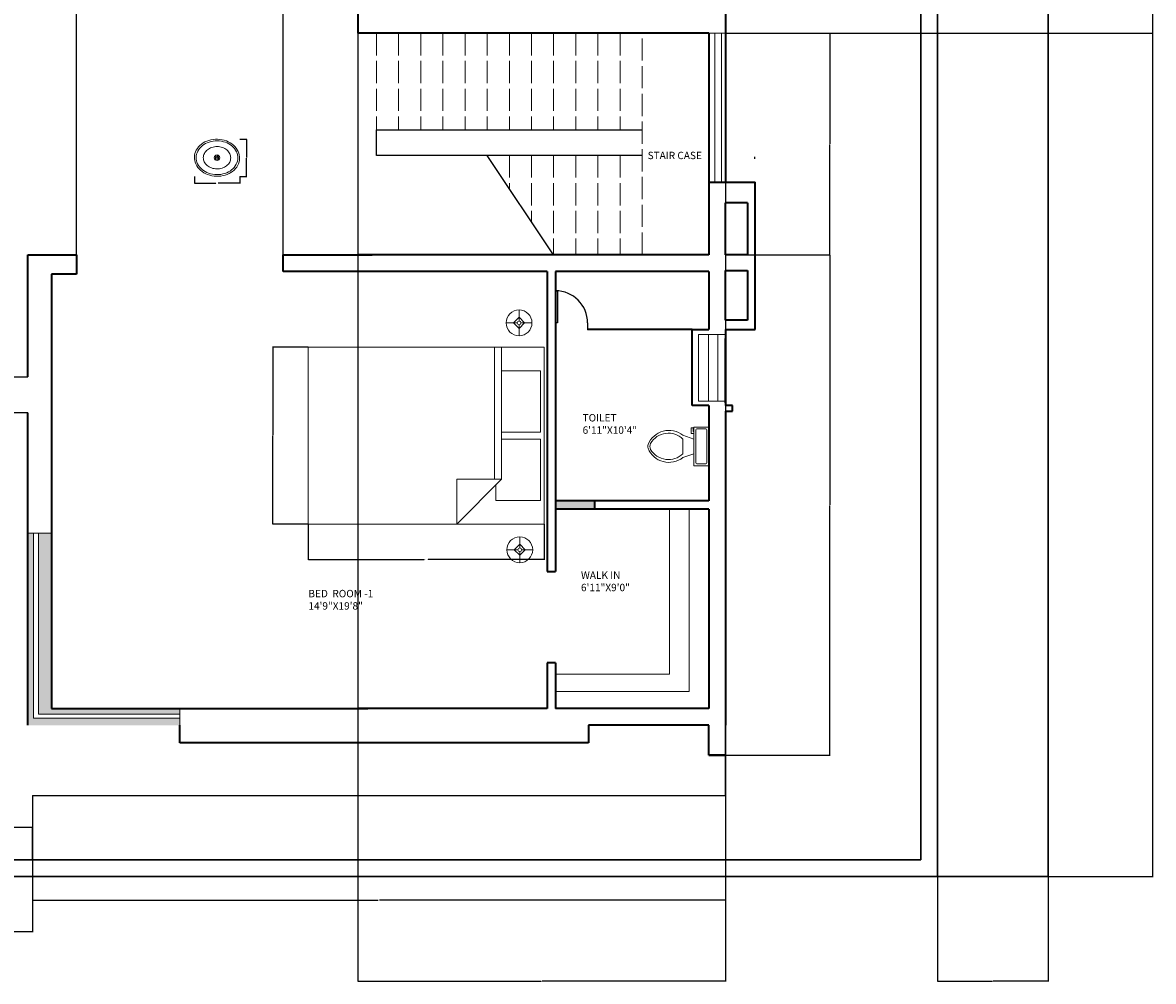
# Model space of a CAD drawing. Units: inches. Extents: x 727 to 1967, y -579 to 606.
# Tile 4 of 5: x 1355 to 1967, y -579 to -60. Entities that reach past the tile are written whole.
import ezdxf

# ---------------------------------------------------------------- set-up
doc = ezdxf.new("R2010")
doc.units = ezdxf.units.IN
doc.header["$MEASUREMENT"] = 0
doc.linetypes.add('ACAD_ISO02W100', pattern=[15, 12, -3])
for name, color, linetype, lineweight in [('A-ANNO-DIMS', 2, 'Continuous', 18), ('A-AREA-IDEN', 7, 'Continuous', 18), ('A-DOOR', 3, 'Continuous', 25), ('A-FLOR-CABT', 8, 'Continuous', 18), ('A-FLOR-EXT', 7, 'Continuous', 25), ('A-FLOR-FIXT', 9, 'Continuous', 18), ('A-FLOR-STRS', 7, 'Continuous', 25), ('A-FLOR-STRS-OVHD', 8, 'ACAD_ISO02W100', 18), ('A-FURN', 8, 'Continuous', 18), ('A-GLAZ', 4, 'Continuous', 18), ('A-GLAZ-PATT', 9, 'Continuous', 13), ('A-WALL', 7, 'Continuous', 35), ('A-WALL-PATT', 9, 'Continuous', 13), ('C-PROP', 7, 'Continuous', 30)]:
    doc.layers.add(name, color=color, linetype=linetype, lineweight=lineweight)
doc.styles.get("Standard").update_dxf_attribs({"font": 'arial.ttf'})
doc.dimstyles.get("Standard").update_dxf_attribs({"dimtxt": 0.18, "dimasz": 0.18, "dimexe": 0.18, "dimexo": 0.0625, "dimgap": 0.09, "dimtad": 0, "dimtih": 1, "dimtoh": 1, "dimdec": 4, "dimzin": 0, "dimdsep": 46, "dimtxsty": 'Standard', "dimcen": 0.09, "dimadec": 0, "dimazin": 0, "dimtfac": 1, "dimtdec": 4, "dimtofl": 0, "dimtmove": 0, "dimatfit": 3, "dimfxl": 1, "dimtolj": 1, "dimtzin": 0, "dimarcsym": 0})

# ---------------------------------------------------------------- blocks, each defined once
blk = doc.blocks.new('*U2')
for p, q in [((0, 0), (0, -6)), ((28, 0), (28, -6))]:
    blk.add_line(p, q)
blk.add_lwpolyline([(0, 0), (0, 28), (1.75, 28), (1.75, 0)], close=True)
blk.add_arc((0, 0), 28, 0, 90)
blk = doc.blocks.new('Bed - Queen')
for p, q in [((0, -80.00003), (0, 0)), ((0, 0), (59.99999, 0)), ((59.99999, 0), (59.99999, -80.00003)), ((7.99999, -1.2), (28.79998, -1.2)), ((7.99999, -14.4), (7.99999, -1.2)), ((28.79998, -1.2), (28.79998, -14.4)), ((31.19999, -1.2), (51.99999, -1.2)), ((31.19999, -14.4), (31.19999, -1.2)), ((51.99999, -1.2), (51.99999, -16.4)), ((0, -14.4), (44.8, -14.4)), ((59.99999, -29.6), (44.8, -14.4)), ((44.8, -14.4), (44.8, -29.6)), ((44.8, -16.8), (0, -16.8)), ((51.99999, -16.4), (46.79936, -16.4)), ((44.8, -29.6), (59.99999, -29.6)), ((59.99999, -80.00003), (0, -80.00003))]:
    blk.add_line(p, q)
blk = doc.blocks.new('Toilet - top')
for p, q in [((9.5, -6), (9.5, -2)), ((-10, -8.5), (-8, -8.5)), ((-10, -9.5), (-10, -8.5)), ((-7, -9.5), (-10, -9.5)), ((-8, -8.5), (-8, -8)), ((-7, -8), (-7, -9.5)), ((-4, -8), (-6, -14)), ((4, -8), (6, -14)), ((4, -14), (-4, -14))]:
    blk.add_line(p, q)
blk.add_lwpolyline([(10.5, -8), (10.5, 0), (-10.5, 0), (-10.5, -8)], close=True)
for points in [[(-9.5, -2), (-9.5, -6)], [(8.5, -1), (-8.5, -1)], [(-8.5, -7), (8.5, -7)]]:
    blk.add_lwpolyline(points)
for centre, radius, start, end in [((-8.62, -1.88), 0.884, 81.8699, 188.1301), ((-8.62, -6.12), 0.884, 171.8699, 278.1301), ((8.62, -1.88), 0.884, 351.8699, 98.1301), ((8.62, -6.12), 0.884, 261.8699, 8.1301), ((3.52, -21.58), 12.17, 141.46911, 247.97143), ((4.2, -21.82), 11.33, 136.36773, 238.94682), ((-3.52, -21.58), 12.17, 292.02843, 38.53071), ((-4.2, -21.82), 11.33, 301.05301, 43.63209), ((0, -27.88), 4, 245.73182, 294.26817), ((0, -29), 4, 254.86053, 285.13947)]:
    blk.add_arc(centre, radius, start, end)
blk = doc.blocks.new('Sink - Oval top')
for p, q in [((-1, 0), (1, 0)), ((0, 1), (0, -1))]:
    blk.add_line(p, q)
for points in [[(-12.23, 0.39, 0.117634), (-11.46, -3.36, 0.104469), (-8.88, -6.8, 0.090016), (-5.08, -9.07, 0.08192), (-0.32, -10.02, 0.08192), (4.49, -9.38, 0.090016), (8.42, -7.36, 0.104469), (11.22, -4.09, 0.117634), (12.23, -0.39, 0.117634), (11.46, 3.36, 0.104469), (8.88, 6.8, 0.090016), (5.08, 9.07, 0.08192), (0.32, 10.02, 0.08192), (-4.49, 9.38, 0.090016), (-8.42, 7.36, 0.104469), (-11.22, 4.09, 0.117634)], [(-11.29, 0.16, 0.118622), (-10.52, -3.25, 0.104678), (-8.07, -6.36, 0.089562), (-4.54, -8.37, 0.081185), (-0.13, -9.15, 0.081185), (4.3, -8.49, 0.089562), (7.89, -6.58, 0.104678), (10.42, -3.55, 0.118622), (11.29, -0.16, 0.118622), (10.52, 3.25, 0.104678), (8.07, 6.36, 0.089562), (4.54, 8.37, 0.081185), (0.13, 9.15, 0.081185), (-4.3, 8.49, 0.089562), (-7.89, 6.58, 0.104678), (-10.42, 3.55, 0.118622)], [(-7.42, 0.08, 0.118283), (-6.91, -2.17, 0.104607), (-5.29, -4.21, 0.089718), (-2.97, -5.53, 0.081436), (-0.07, -6.04, 0.081436), (2.84, -5.59, 0.089718), (5.2, -4.33, 0.104607), (6.86, -2.32, 0.118283), (7.42, -0.08, 0.118283), (6.91, 2.17, 0.104607), (5.29, 4.21, 0.089718), (2.97, 5.53, 0.081436), (0.07, 6.04, 0.081436), (-2.84, 5.59, 0.089718), (-5.2, 4.33, 0.104607), (-6.86, 2.32, 0.118283)]]:
    blk.add_lwpolyline(points, format="xyb", close=True)
for radius in [1.5, 1]:
    blk.add_circle((0, 0), radius)
blk = doc.blocks.new('Lamp - Table')
for p, q in [((0, 7), (0, 1)), ((-1, 0), (-7, 0)), ((0, 3), (-3, 0)), ((-3, 0), (0, -3)), ((3, 0), (0, 3)), ((0, -3), (3, 0)), ((1, 0), (7, 0)), ((0, -1), (0, -7))]:
    blk.add_line(p, q)
for radius in [7, 1]:
    blk.add_circle((0, 0), radius)
blk = doc.blocks.new('*D32')
at = {"layer": 'A-ANNO-DIMS', "color": 0, "lineweight": -2, "transparency": 16777216}
for p, q in [((1509.38, -331.22), (1509.38, -350.5)), ((1637.15, -331.22), (1637.15, -350.5)), ((1509.56, -350.32), (1572.2, -350.32)), ((1636.97, -350.32), (1574.33, -350.32))]:
    blk.add_line(p, q, dxfattribs=at)
at = {"layer": 'A-ANNO-DIMS', "color": 0, "transparency": 16777216}
for points in [[(1509.56, -350.29), (1509.56, -350.35), (1509.38, -350.32)], [(1636.97, -350.29), (1636.97, -350.35), (1637.15, -350.32)]]:
    blk.add_solid(points, dxfattribs=at)
at = {"layer": 'Defpoints', "color": 0, "transparency": 16777216}
for p in [(1509.38, -331.15), (1637.15, -331.15), (1637.15, -350.32)]:
    blk.add_point(p, dxfattribs=at)
at = {"layer": 'A-ANNO-DIMS', "color": 0, "transparency": 16777216, "insert": (1573.27, -350.32), "char_height": 0.18, "attachment_point": 5}
blk.add_mtext('\\A1;QUEEN BED 128', dxfattribs=at)
blk = doc.blocks.new('*D33')
at = {"layer": 'A-ANNO-DIMS', "color": 0, "lineweight": -2, "transparency": 16777216}
for p, q in [((1509.32, -235.33), (1490.04, -235.33)), ((1490.22, -235.51), (1490.22, -283.06)), ((1490.22, -330.97), (1490.22, -283.42)), ((1509.32, -331.15), (1490.04, -331.15))]:
    blk.add_line(p, q, dxfattribs=at)
at = {"layer": 'A-ANNO-DIMS', "color": 0, "transparency": 16777216}
for points in [[(1490.19, -235.51), (1490.25, -235.51), (1490.22, -235.33)], [(1490.19, -330.97), (1490.25, -330.97), (1490.22, -331.15)]]:
    blk.add_solid(points, dxfattribs=at)
at = {"layer": 'Defpoints', "color": 0, "transparency": 16777216}
for p in [(1509.38, -235.33), (1490.22, -331.15), (1509.38, -331.15)]:
    blk.add_point(p, dxfattribs=at)
at = {"layer": 'A-ANNO-DIMS', "color": 0, "transparency": 16777216, "insert": (1490.22, -283.24), "char_height": 0.18, "attachment_point": 5}
blk.add_mtext('\\A1;96', dxfattribs=at)
blk = doc.blocks.new('*D36')
at = {"layer": 'A-ANNO-DIMS', "color": 0, "lineweight": -2, "transparency": 16777216}
for p, q in [((1447.75, -142.98), (1447.75, -146.78)), ((1447.93, -146.6), (1459.4, -146.6)), ((1472.12, -146.6), (1460.65, -146.6)), ((1472.3, -142.98), (1472.3, -146.78))]:
    blk.add_line(p, q, dxfattribs=at)
at = {"layer": 'A-ANNO-DIMS', "color": 0, "transparency": 16777216}
for points in [[(1447.93, -146.57), (1447.93, -146.63), (1447.75, -146.6)], [(1472.12, -146.57), (1472.12, -146.63), (1472.3, -146.6)]]:
    blk.add_solid(points, dxfattribs=at)
at = {"layer": 'Defpoints', "color": 0, "transparency": 16777216}
for p in [(1447.75, -142.92), (1472.3, -142.92), (1472.3, -146.6)]:
    blk.add_point(p, dxfattribs=at)
at = {"layer": 'A-ANNO-DIMS', "color": 0, "transparency": 16777216, "insert": (1460.02, -146.6), "char_height": 0.18, "attachment_point": 5}
blk.add_mtext('\\A1;BASIN 25', dxfattribs=at)
blk = doc.blocks.new('*D37')
at = {"layer": 'A-ANNO-DIMS', "color": 0, "lineweight": -2, "transparency": 16777216}
for p, q in [((1472.36, -122.79), (1476.16, -122.79)), ((1475.98, -122.97), (1475.98, -132.67)), ((1475.98, -142.74), (1475.98, -133.04)), ((1472.36, -142.92), (1476.16, -142.92))]:
    blk.add_line(p, q, dxfattribs=at)
at = {"layer": 'A-ANNO-DIMS', "color": 0, "transparency": 16777216}
for points in [[(1475.95, -122.97), (1476.01, -122.97), (1475.98, -122.79)], [(1475.95, -142.74), (1476.01, -142.74), (1475.98, -142.92)]]:
    blk.add_solid(points, dxfattribs=at)
at = {"layer": 'Defpoints', "color": 0, "transparency": 16777216}
for p in [(1472.3, -122.79), (1475.98, -122.79), (1472.3, -142.92)]:
    blk.add_point(p, dxfattribs=at)
at = {"layer": 'A-ANNO-DIMS', "color": 0, "transparency": 16777216, "insert": (1475.98, -132.85), "char_height": 0.18, "attachment_point": 5}
blk.add_mtext('\\A1;20', dxfattribs=at)
blk = doc.blocks.new('*D39')
at = {"layer": 'A-ANNO-DIMS', "color": 0, "lineweight": -2, "transparency": 16777216}
for p, q in [((1910.24, 548.89), (1966.96, 548.89)), ((1966.78, 548.71), (1966.78, 13.72)), ((1966.78, -521.63), (1966.78, 13.36)), ((1910.24, -521.81), (1966.96, -521.81))]:
    blk.add_line(p, q, dxfattribs=at)
at = {"layer": 'A-ANNO-DIMS', "color": 0, "transparency": 16777216}
for points in [[(1966.75, 548.71), (1966.81, 548.71), (1966.78, 548.89)], [(1966.75, -521.63), (1966.81, -521.63), (1966.78, -521.81)]]:
    blk.add_solid(points, dxfattribs=at)
at = {"layer": 'Defpoints', "color": 0, "transparency": 16777216}
for p in [(1910.18, 548.89), (1966.78, 548.89), (1910.18, -521.81)]:
    blk.add_point(p, dxfattribs=at)
at = {"layer": 'A-ANNO-DIMS', "color": 0, "transparency": 16777216, "insert": (1966.78, 13.54), "char_height": 0.18, "attachment_point": 5}
blk.add_mtext('\\A1;1070.7', dxfattribs=at)
blk = doc.blocks.new('*D44')
at = {"layer": 'A-ANNO-DIMS', "color": 0, "lineweight": -2, "transparency": 16777216}
for p, q in [((1850.18, -521.87), (1850.18, -578.59)), ((1910.18, -521.87), (1910.18, -578.59)), ((1850.36, -578.41), (1879.96, -578.41)), ((1910, -578.41), (1880.4, -578.41))]:
    blk.add_line(p, q, dxfattribs=at)
at = {"layer": 'A-ANNO-DIMS', "color": 0, "transparency": 16777216}
for points in [[(1850.36, -578.38), (1850.36, -578.44), (1850.18, -578.41)], [(1910, -578.38), (1910, -578.44), (1910.18, -578.41)]]:
    blk.add_solid(points, dxfattribs=at)
at = {"layer": 'Defpoints', "color": 0, "transparency": 16777216}
for p in [(1850.18, -521.81), (1910.18, -521.81), (1910.18, -578.41)]:
    blk.add_point(p, dxfattribs=at)
at = {"layer": 'A-ANNO-DIMS', "color": 0, "transparency": 16777216, "insert": (1880.18, -578.41), "char_height": 0.18, "attachment_point": 5}
blk.add_mtext('\\A1;60', dxfattribs=at)
blk = doc.blocks.new('*D50')
at = {"layer": 'A-ANNO-DIMS', "color": 0, "lineweight": -2, "transparency": 16777216}
for p, q in [((971.46, -495.19), (971.46, -551.9)), ((1360.08, -495.19), (1360.08, -551.9)), ((971.64, -551.72), (1165.38, -551.72)), ((1359.9, -551.72), (1166.17, -551.72))]:
    blk.add_line(p, q, dxfattribs=at)
at = {"layer": 'A-ANNO-DIMS', "color": 0, "transparency": 16777216}
for points in [[(971.64, -551.69), (971.64, -551.75), (971.46, -551.72)], [(1359.9, -551.69), (1359.9, -551.75), (1360.08, -551.72)]]:
    blk.add_solid(points, dxfattribs=at)
at = {"layer": 'Defpoints', "color": 0, "transparency": 16777216}
for p in [(971.46, -495.12), (1360.08, -495.12), (971.46, -551.72)]:
    blk.add_point(p, dxfattribs=at)
at = {"layer": 'A-ANNO-DIMS', "color": 0, "transparency": 16777216, "insert": (1165.77, -551.72), "char_height": 0.18, "attachment_point": 5}
blk.add_mtext('\\A1;388.6', dxfattribs=at)
blk = doc.blocks.new('*D51')
at = {"layer": 'A-ANNO-DIMS', "color": 0, "lineweight": -2, "transparency": 16777216}
for p, q in [((1360.08, -478.08), (1360.08, -534.8)), ((1735.35, -478.08), (1735.35, -534.8)), ((1360.26, -534.62), (1547.32, -534.62)), ((1735.17, -534.62), (1548.11, -534.62))]:
    blk.add_line(p, q, dxfattribs=at)
at = {"layer": 'A-ANNO-DIMS', "color": 0, "transparency": 16777216}
for points in [[(1360.26, -534.59), (1360.26, -534.65), (1360.08, -534.62)], [(1735.17, -534.59), (1735.17, -534.65), (1735.35, -534.62)]]:
    blk.add_solid(points, dxfattribs=at)
at = {"layer": 'Defpoints', "color": 0, "transparency": 16777216}
for p in [(1360.08, -478.02), (1735.35, -478.02), (1360.08, -534.62)]:
    blk.add_point(p, dxfattribs=at)
at = {"layer": 'A-ANNO-DIMS', "color": 0, "transparency": 16777216, "insert": (1547.71, -534.62), "char_height": 0.18, "attachment_point": 5}
blk.add_mtext('\\A1;375.3', dxfattribs=at)
blk = doc.blocks.new('*D52')
at = {"layer": 'A-ANNO-DIMS', "color": 0, "lineweight": -2, "transparency": 16777216}
for p, q in [((1735.41, -65.48), (1792.13, -65.48)), ((1791.95, -65.66), (1791.95, -125.3)), ((1791.95, -185.3), (1791.95, -125.67)), ((1735.41, -185.48), (1792.13, -185.48))]:
    blk.add_line(p, q, dxfattribs=at)
at = {"layer": 'A-ANNO-DIMS', "color": 0, "transparency": 16777216}
for points in [[(1791.92, -65.66), (1791.98, -65.66), (1791.95, -65.48)], [(1791.92, -185.3), (1791.98, -185.3), (1791.95, -185.48)]]:
    blk.add_solid(points, dxfattribs=at)
at = {"layer": 'Defpoints', "color": 0, "transparency": 16777216}
for p in [(1735.35, -65.48), (1735.35, -185.48), (1791.95, -185.48)]:
    blk.add_point(p, dxfattribs=at)
at = {"layer": 'A-ANNO-DIMS', "color": 0, "transparency": 16777216, "insert": (1791.95, -125.48), "char_height": 0.18, "attachment_point": 5}
blk.add_mtext('\\A1;120', dxfattribs=at)
blk = doc.blocks.new('*D53')
at = {"layer": 'A-ANNO-DIMS', "color": 0, "lineweight": -2, "transparency": 16777216}
for p, q in [((1735.41, -185.48), (1792.13, -185.48)), ((1791.95, -185.66), (1791.95, -320.65)), ((1791.95, -456), (1791.95, -321.02)), ((1735.41, -456.18), (1792.13, -456.18))]:
    blk.add_line(p, q, dxfattribs=at)
at = {"layer": 'A-ANNO-DIMS', "color": 0, "transparency": 16777216}
for points in [[(1791.92, -185.66), (1791.98, -185.66), (1791.95, -185.48)], [(1791.92, -456), (1791.98, -456), (1791.95, -456.18)]]:
    blk.add_solid(points, dxfattribs=at)
at = {"layer": 'Defpoints', "color": 0, "transparency": 16777216}
for p in [(1735.35, -185.48), (1735.35, -456.18), (1791.95, -456.18)]:
    blk.add_point(p, dxfattribs=at)
at = {"layer": 'A-ANNO-DIMS', "color": 0, "transparency": 16777216, "insert": (1791.95, -320.83), "char_height": 0.18, "attachment_point": 5}
blk.add_mtext('\\A1;270.7', dxfattribs=at)
blk = doc.blocks.new('*D60')
at = {"layer": 'A-ANNO-DIMS', "color": 0, "lineweight": -2, "transparency": 16777216}
for p, q in [((1383.91, -185.42), (1383.91, 605.67)), ((1384.09, 605.49), (1439.47, 605.49)), ((1495.75, 605.49), (1440.38, 605.49)), ((1495.93, -185.42), (1495.93, 605.67))]:
    blk.add_line(p, q, dxfattribs=at)
at = {"layer": 'A-ANNO-DIMS', "color": 0, "transparency": 16777216}
for points in [[(1384.09, 605.52), (1384.09, 605.46), (1383.91, 605.49)], [(1495.75, 605.52), (1495.75, 605.46), (1495.93, 605.49)]]:
    blk.add_solid(points, dxfattribs=at)
at = {"layer": 'Defpoints', "color": 0, "transparency": 16777216}
for p in [(1495.93, 605.49), (1383.91, -185.48), (1495.93, -185.48)]:
    blk.add_point(p, dxfattribs=at)
at = {"layer": 'A-ANNO-DIMS', "color": 0, "transparency": 16777216, "insert": (1439.92, 605.49), "char_height": 0.18, "attachment_point": 5}
blk.add_mtext('\\A1;112.02', dxfattribs=at)
blk = doc.blocks.new('*D67')
at = {"layer": 'A-ANNO-DIMS', "color": 0, "lineweight": -2, "transparency": 16777216}
for p, q in [((1735.41, -14.75), (1966.96, -14.75)), ((1966.78, -14.93), (1966.78, -39.94)), ((1966.78, -65.3), (1966.78, -40.3)), ((1735.41, -65.48), (1966.96, -65.48))]:
    blk.add_line(p, q, dxfattribs=at)
at = {"layer": 'A-ANNO-DIMS', "color": 0, "transparency": 16777216}
for points in [[(1966.75, -14.93), (1966.81, -14.93), (1966.78, -14.75)], [(1966.75, -65.3), (1966.81, -65.3), (1966.78, -65.48)]]:
    blk.add_solid(points, dxfattribs=at)
at = {"layer": 'Defpoints', "color": 0, "transparency": 16777216}
for p in [(1735.35, -14.75), (1735.35, -65.48), (1966.78, -65.48)]:
    blk.add_point(p, dxfattribs=at)
at = {"layer": 'A-ANNO-DIMS', "color": 0, "transparency": 16777216, "insert": (1966.78, -40.12), "char_height": 0.18, "attachment_point": 5}
blk.add_mtext('\\A1;50.73', dxfattribs=at)
blk = doc.blocks.new('*D68')
at = {"layer": 'A-ANNO-DIMS', "color": 0, "lineweight": -2, "transparency": 16777216}
for p, q in [((1536.35, -65.55), (1536.35, -578.59)), ((1735.35, -65.55), (1735.35, -578.59)), ((1536.53, -578.41), (1635.57, -578.41)), ((1735.17, -578.41), (1636.13, -578.41))]:
    blk.add_line(p, q, dxfattribs=at)
at = {"layer": 'A-ANNO-DIMS', "color": 0, "transparency": 16777216}
for points in [[(1536.53, -578.38), (1536.53, -578.44), (1536.35, -578.41)], [(1735.17, -578.38), (1735.17, -578.44), (1735.35, -578.41)]]:
    blk.add_solid(points, dxfattribs=at)
at = {"layer": 'Defpoints', "color": 0, "transparency": 16777216}
for p in [(1536.35, -65.48), (1735.35, -65.48), (1735.35, -578.41)]:
    blk.add_point(p, dxfattribs=at)
at = {"layer": 'A-ANNO-DIMS', "color": 0, "transparency": 16777216, "insert": (1635.85, -578.41), "char_height": 0.18, "attachment_point": 5}
blk.add_mtext('\\A1;199', dxfattribs=at)

msp = doc.modelspace()

# ---------------------------------------------------------------- hatches: boundary and pattern name
at = {"layer": 'A-GLAZ-PATT'}
h = msp.add_hatch(color=256, dxfattribs=at)
h.dxf.hatch_style = 1
h.paths.add_polyline_path([(1370.4043, -336.0425), (1363.3494, -336.0425), (1363.3494, -434.0523), (1439.8357, -434.0523), (1439.8357, -430.9849), (1370.4043, -430.9849)], flags=17)
h.paths.add_polyline_path([(1360.6917, -336.0425), (1357.6449, -336.0425), (1357.6449, -439.9849), (1439.8357, -439.9849), (1439.8357, -436.1404), (1360.6917, -436.1404)])
at = {"layer": 'A-WALL-PATT'}
h = msp.add_hatch(color=256, dxfattribs=at)
h.dxf.hatch_style = 1
h.paths.add_polyline_path([(1643.3463, -318.4849), (1643.3463, -322.9849), (1664.7357, -322.9849), (1664.7357, -318.4849)])

# ---------------------------------------------------------------- linework, layer by layer
at = {"layer": 'A-FLOR-CABT'}
for p, q in [((1705.0854, -412.3686), (1705.0854, -322.9849)), ((1705.0854, -322.9849), (1726.3463, -322.9849)), ((1726.3463, -322.9849), (1715.7158, -322.9849)), ((1715.7158, -322.9849), (1715.7158, -421.7787)), ((1643.3463, -412.3686), (1705.0854, -412.3686)), ((1715.7158, -421.7787), (1643.3463, -421.7787))]:
    msp.add_line(p, q, dxfattribs=at)
at = {"layer": 'A-FLOR-EXT'}
for p, q in [((1301.8463, -251.4849), (1357.6449, -251.4849)), ((1357.6449, -270.8759), (971.4628, -270.8759)), ((1735.3463, -478.0203), (1735.3463, -439.9849)), ((1360.0813, -478.0203), (1360.0813, -495.1242)), ((1360.0813, -478.0203), (1735.3463, -478.0203)), ((971.4628, -495.1242), (1360.0813, -495.1242)), ((1360.0813, -512.8103), (1360.0813, -495.1242)), ((1360.0813, -495.1242), (1360.0813, -521.8103))]:
    msp.add_line(p, q, dxfattribs=at)
at = {"layer": 'A-FLOR-STRS'}
for p, q in [((1546.3463, -131.6287), (1546.3463, -117.7515)), ((1546.3463, -117.7515), (1690.3463, -117.7515)), ((1690.3463, -131.6287), (1546.3463, -131.6287)), ((1642.3463, -185.4849), (1606.3463, -131.6287))]:
    msp.add_line(p, q, dxfattribs=at)
at = {"layer": 'A-FLOR-STRS-OVHD'}
for p, q in [((1546.3463, -65.4849), (1546.3463, -131.6287)), ((1558.3463, -65.4849), (1558.3463, -117.7515)), ((1570.3463, -65.4849), (1570.3463, -117.7515)), ((1582.3463, -65.4849), (1582.3463, -117.7515)), ((1594.3463, -65.4849), (1594.3463, -117.7515)), ((1606.3463, -65.4849), (1606.3463, -117.7515)), ((1618.3463, -65.4849), (1618.3463, -117.7515)), ((1630.3463, -65.4849), (1630.3463, -117.7515)), ((1642.3463, -65.4849), (1642.3463, -117.7515)), ((1654.3463, -65.4849), (1654.3463, -117.7515)), ((1666.3463, -65.4849), (1666.3463, -117.7515)), ((1678.3463, -65.4849), (1678.3463, -117.7515)), ((1690.3463, -68.2669), (1690.3463, -188.2669)), ((1618.3463, -131.6287), (1618.3463, -149.5808)), ((1630.3463, -131.6287), (1630.3463, -167.5328)), ((1642.3463, -131.6287), (1642.3463, -185.4849)), ((1654.3463, -131.6287), (1654.3463, -185.4849)), ((1666.3463, -131.6287), (1666.3463, -185.4849)), ((1678.3463, -131.6287), (1678.3463, -185.4849))]:
    msp.add_line(p, q, dxfattribs=at)
at = {"layer": 'A-GLAZ'}
for p, q in [((1726.3463, -65.4849), (1735.3463, -65.4849)), ((1729.7207, -146.0061), (1729.7207, -65.4849)), ((1735.3463, -65.4849), (1733.3258, -65.4849)), ((1733.3258, -65.4849), (1733.3258, -146.0061)), ((1733.3258, -146.0061), (1729.7207, -146.0061)), ((1720.8368, -264.5359), (1720.8368, -228.4847)), ((1720.8368, -228.4847), (1735.3463, -228.4847)), ((1731.284, -228.4847), (1726.1819, -228.4847)), ((1726.1819, -228.4847), (1726.1819, -264.5359)), ((1731.284, -264.5359), (1731.284, -228.4847)), ((1735.3463, -264.5359), (1720.8368, -264.5359)), ((1370.4043, -336.0425), (1357.6449, -336.0425)), ((1360.6917, -336.0425), (1360.6917, -436.1404)), ((1363.3494, -434.0523), (1363.3494, -336.0425)), ((1363.3494, -336.0425), (1363.3494, -336.0425)), ((1370.4043, -430.9849), (1370.4043, -336.0425)), ((1439.8357, -434.0523), (1363.3494, -434.0523)), ((1439.8357, -430.9849), (1370.4043, -430.9849)), ((1439.8357, -439.9849), (1439.8357, -430.9849)), ((1439.8357, -435.4849), (1439.8357, -434.0523)), ((1360.6917, -436.1404), (1439.8357, -436.1404)), ((1439.8357, -436.1404), (1439.8357, -435.4849))]:
    msp.add_line(p, q, dxfattribs=at)
at = {"layer": 'A-WALL'}
for p, q in [((1735.3463, 209.3543), (1735.3463, -146.0061)), ((1536.3463, 114.5151), (1536.3463, -65.4849)), ((1726.3463, -65.4849), (1536.3463, -65.4849)), ((1726.3463, -65.4849), (1726.3463, -142.1959)), ((1751.474, -132.9361), (1750.9882, -132.9361)), ((1750.9882, -132.9361), (1751.474, -132.9361)), ((1726.3463, -137.9716), (1726.3463, -185.4849)), ((1726.3463, -146.0061), (1751.474, -146.0061)), ((1751.474, -225.839), (1751.474, -146.0061)), ((1747.279, -157.2135), (1735.3463, -157.2135)), ((1735.3463, -185.4849), (1735.3463, -157.2135)), ((1747.279, -157.2135), (1747.279, -185.4849)), ((1357.6449, -185.4849), (1377.7899, -185.4849)), ((1357.6449, -251.4849), (1357.6449, -185.4849)), ((1377.7899, -185.4849), (1383.9141, -185.4849)), ((1383.9141, -185.4849), (1383.9141, -195.8509)), ((1495.9329, -194.4849), (1495.9329, -185.4849)), ((1495.9329, -185.4849), (1544.0588, -185.4849)), ((1726.3463, -185.4849), (1536.3463, -185.4849)), ((1747.279, -185.4849), (1735.3463, -185.4849)), ((1383.9141, -195.8509), (1370.4043, -195.8509)), ((1370.4043, -195.8509), (1370.4043, -430.9849)), ((1536.3463, -194.4849), (1495.9329, -194.4849)), ((1638.8463, -194.4849), (1536.3463, -194.4849)), ((1638.8463, -194.4849), (1638.8463, -356.7647)), ((1726.3463, -194.4849), (1643.3463, -194.4849)), ((1643.3463, -194.4849), (1643.3463, -356.7647)), ((1726.3463, -194.4849), (1726.3463, -225.839)), ((1735.3463, -220.6908), (1735.3463, -193.9588)), ((1735.3463, -193.9588), (1747.279, -193.9588)), ((1747.279, -193.9588), (1747.279, -220.6908)), ((1673.6603, -225.839), (1660.7507, -225.839)), ((1717.3505, -225.839), (1673.6603, -225.839)), ((1717.3505, -240.1592), (1717.3505, -225.839)), ((1717.3505, -225.839), (1726.3463, -225.839)), ((1747.279, -220.6908), (1735.3463, -220.6908)), ((1735.3463, -225.839), (1735.3463, -266.9698)), ((1735.3463, -225.839), (1751.474, -225.839)), ((1735.3463, -265.4456), (1735.3463, -230.6189)), ((1717.3505, -266.9698), (1717.3505, -240.1592)), ((1726.3463, -266.9698), (1717.3505, -266.9698)), ((1726.3463, -266.9698), (1726.3463, -318.4849)), ((1739.2524, -266.9698), (1735.3463, -266.9698)), ((1739.2524, -269.9272), (1739.2524, -266.9698)), ((1357.6449, -439.9849), (1357.6449, -270.8759)), ((1735.3463, -269.9272), (1739.2524, -269.9272)), ((1735.3463, -269.9272), (1735.3463, -439.9849)), ((1726.3463, -318.4849), (1643.3463, -318.4849)), ((1726.3463, -322.9849), (1643.3463, -322.9849)), ((1664.7357, -322.9849), (1664.7357, -318.4849)), ((1726.3463, -322.9849), (1726.3463, -430.9849)), ((1638.8463, -356.7647), (1643.3463, -356.7647)), ((1643.3463, -406.1754), (1638.8463, -406.1754)), ((1638.8463, -406.1754), (1638.8463, -430.9849)), ((1643.3463, -406.1754), (1643.3463, -430.9849)), ((1370.4043, -430.9849), (1541.6244, -430.9849)), ((1638.8463, -430.9849), (1536.3463, -430.9849)), ((1726.3463, -430.9849), (1643.3463, -430.9849)), ((1439.8357, -449.4649), (1439.8357, -439.9849)), ((1726.3463, -439.9849), (1661.169, -439.9849)), ((1661.169, -439.9849), (1661.169, -449.4649)), ((1726.3463, -456.1835), (1726.3463, -439.9849)), ((1661.169, -449.4649), (1439.8357, -449.4649)), ((1726.3463, -456.1835), (1735.3463, -456.1835)), ((1735.3463, -456.1835), (1726.3463, -456.1835))]:
    msp.add_line(p, q, dxfattribs=at)
at = {"layer": 'C-PROP'}
for p, q in [((1910.1781, 548.8891), (1910.1781, -521.8103)), ((1850.1781, 392.0151), (1850.1781, -521.8103)), ((1841.1781, 383.0151), (1841.1781, -512.8103)), ((1841.1781, -512.8103), (852.5815, -512.8103)), ((1850.1781, -521.8103), (843.5815, -521.8103)), ((1850.1781, -521.8103), (1910.1781, -521.8103))]:
    msp.add_line(p, q, dxfattribs=at)

# ---------------------------------------------------------------- block references
at = {"layer": 'A-DOOR', "xscale": 0.6215854176028623, "yscale": 0.6215854176028623, "zscale": 0.6215854176028623}
msp.add_blockref('*U2', (1643.3463, -222.2862), dxfattribs=at)
at = {"layer": 'A-FLOR-FIXT'}
msp.add_blockref('Sink - Oval top', (1460.0242, -132.8537), dxfattribs=at)
at = {"layer": 'A-FLOR-FIXT', "rotation": 270.0000413122306}
msp.add_blockref('Toilet - top', (1726.3463, -289.0737), dxfattribs=at)
at = {"layer": 'A-FURN'}
for p in [(1623.6056, -222.2227), (1623.9845, -345.0114)]:
    msp.add_blockref('Lamp - Table', p, dxfattribs=at)
at = {"layer": 'A-FURN', "xscale": 1.597075037824208, "yscale": 1.597075037824208, "zscale": 1.597075037824208, "rotation": 270}
msp.add_blockref('Bed - Queen', (1637.1496, -235.3305), dxfattribs=at)

# ---------------------------------------------------------------- texts
at = {"layer": 'A-AREA-IDEN', "char_height": 4, "attachment_point": 1}
for s, insert in [('STAIR CASE', (1693.2317, -129.6213)), ('TOILET\\P6\'11"X10\'4"', (1658.0191, -271.5806)), ('WALK IN\\P6\'11"X9\'0"', (1657.1456, -356.7647)), ('BED  ROOM -1\\P14\'9"X19\'8"', (1509.5103, -366.7271))]:
    msp.add_mtext_dynamic_manual_height_columns(s, width=588.620786, gutter_width=1, heights=[0], dxfattribs=dict(at, insert=insert))

# ---------------------------------------------------------------- dimensions: what is measured, and where the dimension line sits
at = {"layer": 'A-ANNO-DIMS'}
for base, p1, p2, override, picture, middle in [((1495.9329, 605.4891), (1383.9141, -185.4849), (1495.9329, -185.4849), {"dimdec": 2, "dimlfac": 1, "dimrnd": 0, "dimzin": 0, "dimdsep": 46, "dimlunit": 2}, '*D60', (1439.9235, 605.4891)), ((1735.3463, -578.4103), (1536.3463, -65.4849), (1735.3463, -65.4849), {"dimdec": 0, "dimlfac": 1, "dimrnd": 0, "dimzin": 0, "dimdsep": 46, "dimlunit": 2}, '*D68', (1635.8463, -578.4103)), ((1910.1781, -578.4103), (1850.1781, -521.8103), (1910.1781, -521.8103), {"dimdec": 0, "dimlfac": 1, "dimrnd": 0, "dimzin": 0, "dimdsep": 46, "dimlunit": 2}, '*D44', (1880.1781, -578.4103))]:
    dim = msp.add_linear_dim(base=base, p1=p1, p2=p2, dimstyle='Standard', override=override, dxfattribs=at)
    dim.commit()
    dim.dimension.update_dxf_attribs({"geometry": picture, "text_midpoint": middle})
for base, p1, p2, angle, override, picture, middle in [((1966.7781, 548.8891), (1910.1781, -521.8103), (1910.1781, 548.8891), 90, {"dimdec": 1, "dimlfac": 1, "dimrnd": 0, "dimzin": 0, "dimdsep": 46, "dimlunit": 2}, '*D39', (1966.7781, 13.5394)), ((1966.7781, -65.4849), (1735.3463, -14.7535), (1735.3463, -65.4849), 90, {"dimdec": 2, "dimlfac": 1, "dimrnd": 0, "dimzin": 0, "dimdsep": 46, "dimlunit": 2}, '*D67', (1966.7781, -40.1192)), ((1791.9463, -185.4849), (1735.3463, -65.4849), (1735.3463, -185.4849), 270, {"dimdec": 0, "dimlfac": 1, "dimrnd": 0, "dimzin": 0, "dimdsep": 46, "dimlunit": 2}, '*D52', (1791.9463, -125.4849)), ((1475.9823, -122.7854), (1472.2997, -142.922), (1472.2997, -122.7854), 90, {"dimdec": 0, "dimlfac": 1, "dimrnd": 0, "dimzin": 0, "dimdsep": 46, "dimlunit": 2}, '*D37', (1475.9823, -132.8537)), ((1791.9463, -456.1835), (1735.3463, -185.4849), (1735.3463, -456.1835), 270, {"dimdec": 1, "dimlfac": 1, "dimrnd": 0, "dimzin": 0, "dimdsep": 46, "dimlunit": 2}, '*D53', (1791.9463, -320.8342)), ((1490.2186, -331.155), (1509.3835, -235.3305), (1509.3835, -331.155), 270, {"dimdec": 0, "dimlfac": 1, "dimrnd": 0, "dimzin": 0, "dimdsep": 46, "dimlunit": 2}, '*D33', (1490.2186, -283.2427)), ((1360.0813, -534.6203), (1735.3463, -478.0203), (1360.0813, -478.0203), 180, {"dimdec": 1, "dimlfac": 1, "dimrnd": 0, "dimzin": 0, "dimdsep": 46, "dimlunit": 2}, '*D51', (1547.7138, -534.6203)), ((971.4628, -551.7242), (1360.0813, -495.1242), (971.4628, -495.1242), 180, {"dimdec": 1, "dimlfac": 1, "dimrnd": 0, "dimzin": 0, "dimdsep": 46, "dimlunit": 2}, '*D50', (1165.7721, -551.7242))]:
    dim = msp.add_linear_dim(base=base, p1=p1, p2=p2, angle=angle, dimstyle='Standard', override=override, dxfattribs=at)
    dim.commit()
    dim.dimension.update_dxf_attribs({"geometry": picture, "text_midpoint": middle})
for base, p1, p2, text, picture, middle in [((1472.2997, -146.6047), (1447.7488, -142.922), (1472.2997, -142.922), 'BASIN <>', '*D36', (1460.0242, -146.6047)), ((1637.1496, -350.3199), (1509.3835, -331.155), (1637.1496, -331.155), 'QUEEN BED <>', '*D32', (1573.2666, -350.3199))]:
    dim = msp.add_linear_dim(base=base, p1=p1, p2=p2, text=text, dimstyle='Standard', override={"dimdec": 0, "dimlfac": 1, "dimrnd": 0, "dimzin": 0, "dimdsep": 46, "dimlunit": 2}, dxfattribs=at)
    dim.commit()
    dim.dimension.update_dxf_attribs({"geometry": picture, "text_midpoint": middle})

doc.saveas('drawing.dxf')
